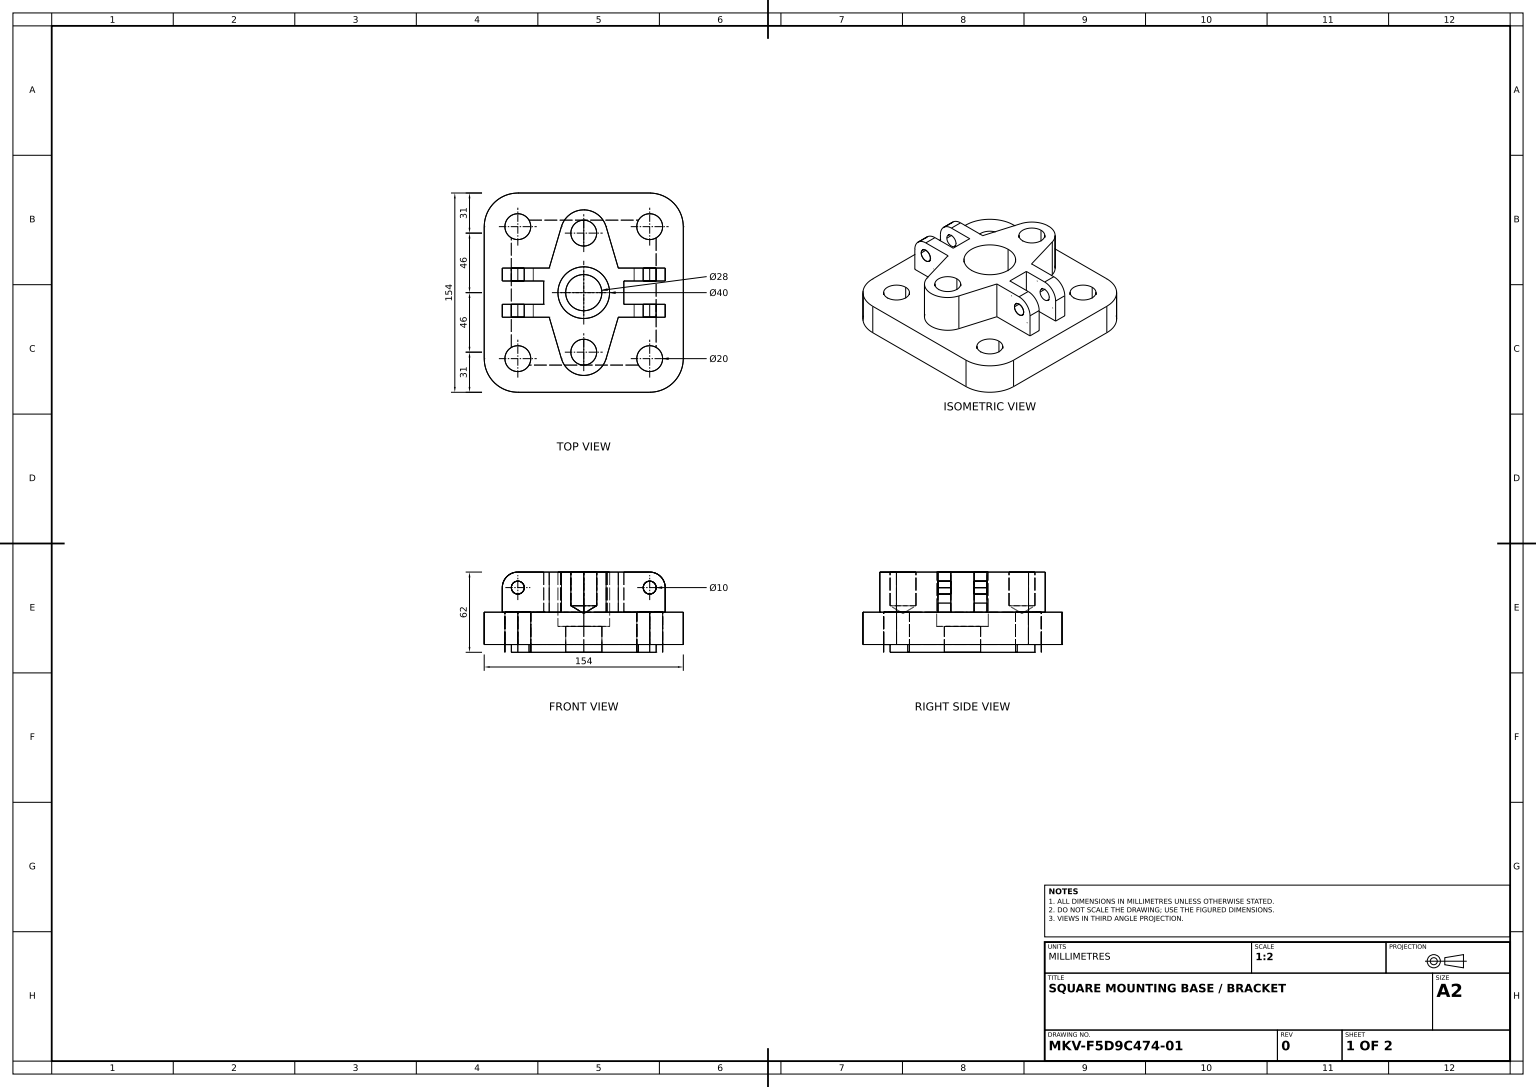
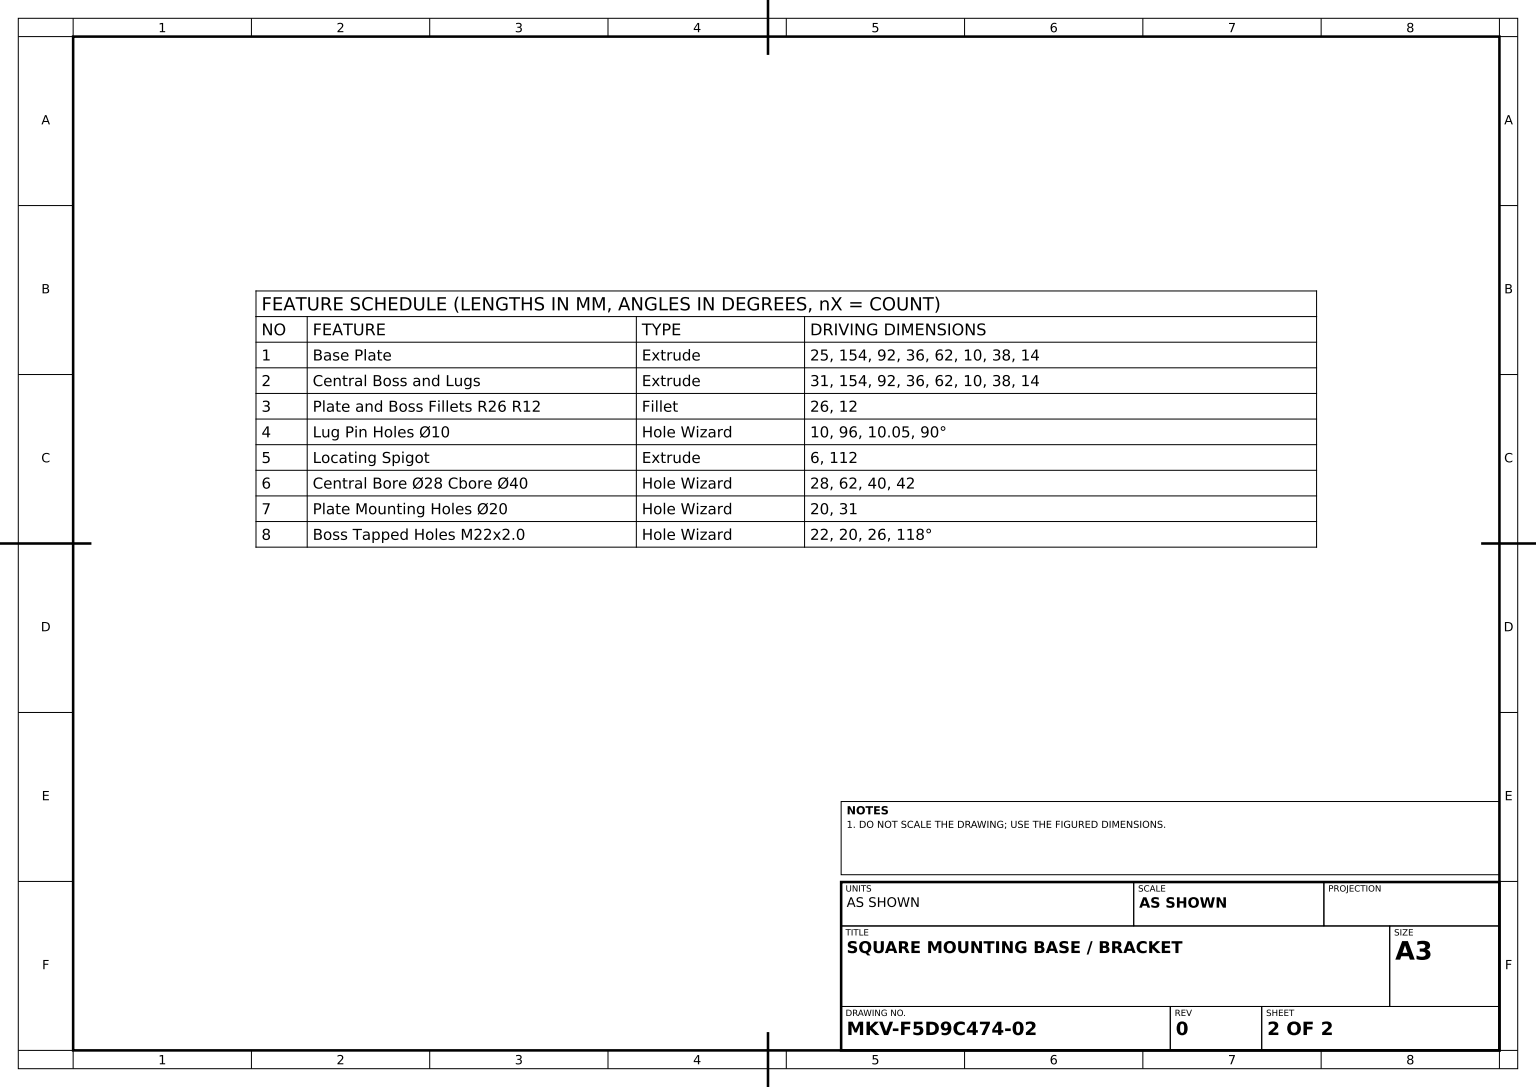
from build123d import *
from OCP.BRepFilletAPI import BRepFilletAPI_MakeFillet

# Parameters (mm, degrees)
PLATE_AND_BOSS_PROFILE_W             = 154
PLATE_AND_BOSS_PROFILE_H             = 154
PLATE_AND_BOSS_PROFILE_R             = 18
BASE_PLATE_DEPTH                     = 25
CENTRAL_START                        = 25
SKETCH1_3_R                          = 18
CENTRAL_BOSS_AND_LUGS_DEPTH          = 31
PLATE_AND_BOSS_FILLETS_R26_R12_R1    = 12
PLATE_AND_BOSS_FILLETS_R26_R12_R2    = 26
LUG_PIN_HOLES_10_D                   = 10
LUG_PIN_HOLES_10_CSINK_D             = 10.05
LUG_PIN_HOLES_10_CSINK_ANGLE         = 90
LOCATING_SPIGOT_PROFILE_112_W        = 112
LOCATING_SPIGOT_PROFILE_112_H        = 112
LOCATING_SPIGOT_DEPTH                = 6
CENTRAL_BORE_28_CBORE_40_D           = 28
CENTRAL_BORE_28_CBORE_40_CBORE_D     = 40
CENTRAL_BORE_28_CBORE_40_CBORE_DEPTH = 42
PLATE_MOUNTING_HOLES_20_D            = 20
BOSS_TAPPED_HOLES_M22X2_0_D          = 20
BOSS_TAPPED_HOLES_M22X2_0_DEPTH      = 26
BOSS_TAPPED_HOLES_M22X2_0_TIP        = 6.00860619


with BuildPart() as part:
    # Plate and Boss Profile → Base Plate (new body)
    # profile 1 of 4: a face of its own
    with BuildSketch(Plane(origin=(0, 0, 0), x_dir=(1, 0, 0), z_dir=(0, 1, 0))):
        Rectangle(PLATE_AND_BOSS_PROFILE_W, PLATE_AND_BOSS_PROFILE_H)
        with BuildLine():
            Line((-26.719653956, 19), (-17.266235066, 51.086956522))
            ThreePointArc((-17.266235066, 51.086956522), (0, 64), (17.266235066, 51.086956522))
            Line((17.266235066, 51.086956522), (26.719653956, 19))
            Line((26.719653956, 19), (63, 19))
            Line((63, 19), (63, 9))
            Line((63, 9), (31, 9))
            Line((31, 9), (31, -9))
            Line((31, -9), (63, -9))
            Line((63, -9), (63, -19))
            Line((63, -19), (26.719653956, -19))
            Line((26.719653956, -19), (17.266235066, -51.086956522))
            ThreePointArc((17.266235066, -51.086956522), (0, -64), (-17.266235066, -51.086956522))
            Line((-17.266235066, -51.086956522), (-26.719653956, -19))
            Line((-26.719653956, -19), (-63, -19))
            Line((-63, -19), (-63, -9))
            Line((-63, -9), (-31, -9))
            Line((-31, -9), (-31, 9))
            Line((-31, 9), (-63, 9))
            Line((-63, 9), (-63, 19))
            Line((-63, 19), (-26.719653956, 19))
        make_face(mode=Mode.SUBTRACT)
    # profile 2 of 4: a face of its own
    with BuildSketch(Plane(origin=(0, 0, 0), x_dir=(1, 0, 0), z_dir=(0, 1, 0))):
        with BuildLine():
            ThreePointArc((18, 46), (-2.569802406, 28.184385624), (-17.266235066, 51.086956522))
            Line((-17.266235066, 51.086956522), (-26.719653956, 19))
            Line((-26.719653956, 19), (-63, 19))
            Line((-63, 19), (-63, 9))
            Line((-63, 9), (-31, 9))
            Line((-31, 9), (-31, -9))
            Line((-31, -9), (-63, -9))
            Line((-63, -9), (-63, -19))
            Line((-63, -19), (-26.719653956, -19))
            Line((-26.719653956, -19), (-17.266235066, -51.086956522))
            ThreePointArc((-17.266235066, -51.086956522), (-2.569802406, -28.184385624), (18, -46))
            ThreePointArc((18, -46), (17.815614376, -48.569802406), (17.266235066, -51.086956522))
            Line((17.266235066, -51.086956522), (26.719653956, -19))
            Line((26.719653956, -19), (63, -19))
            Line((63, -19), (63, -9))
            Line((63, -9), (31, -9))
            Line((31, -9), (31, 9))
            Line((31, 9), (63, 9))
            Line((63, 9), (63, 19))
            Line((63, 19), (26.719653956, 19))
            Line((26.719653956, 19), (17.266235066, 51.086956522))
            ThreePointArc((17.266235066, 51.086956522), (17.815614376, 48.569802406), (18, 46))
        make_face()
    # profile 3 of 4: a face of its own
    with BuildSketch(Plane(origin=(0, 0, 0), x_dir=(1, 0, 0), z_dir=(0, 1, 0))):
        with Locations((0, 46)):
            Circle(PLATE_AND_BOSS_PROFILE_R)
    # profile 4 of 4: a face of its own
    with BuildSketch(Plane(origin=(0, 0, 0), x_dir=(1, 0, 0), z_dir=(0, 1, 0))):
        with Locations((0, -46)):
            Circle(PLATE_AND_BOSS_PROFILE_R)
    extrude(amount=BASE_PLATE_DEPTH)

    # Sketch1_3 → Central Boss and Lugs (add)
    with BuildSketch(Plane(origin=(0, 0, 0), x_dir=(1, 0, 0), z_dir=(0, 1, 0)).offset(CENTRAL_START)):
        with BuildLine():
            ThreePointArc((18, 46), (-2.569802406, 28.184385624), (-17.266235066, 51.086956522))
            Line((-17.266235066, 51.086956522), (-26.719653956, 19))
            Line((-26.719653956, 19), (-63, 19))
            Line((-63, 19), (-63, 9))
            Line((-63, 9), (-31, 9))
            Line((-31, 9), (-31, -9))
            Line((-31, -9), (-63, -9))
            Line((-63, -9), (-63, -19))
            Line((-63, -19), (-26.719653956, -19))
            Line((-26.719653956, -19), (-17.266235066, -51.086956522))
            ThreePointArc((-17.266235066, -51.086956522), (-2.569802406, -28.184385624), (18, -46))
            ThreePointArc((18, -46), (17.815614376, -48.569802406), (17.266235066, -51.086956522))
            Line((17.266235066, -51.086956522), (26.719653956, -19))
            Line((26.719653956, -19), (63, -19))
            Line((63, -19), (63, -9))
            Line((63, -9), (31, -9))
            Line((31, -9), (31, 9))
            Line((31, 9), (63, 9))
            Line((63, 9), (63, 19))
            Line((63, 19), (26.719653956, 19))
            Line((26.719653956, 19), (17.266235066, 51.086956522))
            ThreePointArc((17.266235066, 51.086956522), (17.815614376, 48.569802406), (18, 46))
        make_face()
        with Locations((0, 46)):
            Circle(SKETCH1_3_R)
        with Locations((0, -46)):
            Circle(SKETCH1_3_R)
    extrude(amount=CENTRAL_BOSS_AND_LUGS_DEPTH)

    # Plate and Boss Fillets R26 R12: one fillet with a radius per group of edges: ONE call of the kernel's fillet builder (fillet() takes one radius for all edges)
    plate_and_boss_fillets_r26_r12_edges_1 = [part.edges().sort_by_distance(p)[0] for p in [
        (63, 56, 14),
        (-63, 56, -14),
        (63, 56, -14),
        (-63, 56, 14),
    ]]
    plate_and_boss_fillets_r26_r12_edges_2 = [part.edges().sort_by_distance(p)[0] for p in [
        (77, 12.5, 77),
        (-77, 12.5, 77),
        (-77, 12.5, -77),
        (77, 12.5, -77),
    ]]
    plate_and_boss_fillets_r26_r12 = BRepFilletAPI_MakeFillet(part.part.solid().wrapped)
    for e in plate_and_boss_fillets_r26_r12_edges_1:
        plate_and_boss_fillets_r26_r12.Add(PLATE_AND_BOSS_FILLETS_R26_R12_R1, e.wrapped)
    for e in plate_and_boss_fillets_r26_r12_edges_2:
        plate_and_boss_fillets_r26_r12.Add(PLATE_AND_BOSS_FILLETS_R26_R12_R2, e.wrapped)
    add(Compound.cast(plate_and_boss_fillets_r26_r12.Shape()), mode=Mode.REPLACE)

    # Lug Pin Holes _10 (through all)
    with Locations(Plane.XY.offset(19)):
        with Locations((-51, 44), (51, 44)):
            CounterSinkHole(LUG_PIN_HOLES_10_D / 2, LUG_PIN_HOLES_10_CSINK_D / 2, counter_sink_angle=LUG_PIN_HOLES_10_CSINK_ANGLE)

    # Locating Spigot Profile _112 → Locating Spigot (add)
    with BuildSketch(Plane.XZ):
        Rectangle(LOCATING_SPIGOT_PROFILE_112_W, LOCATING_SPIGOT_PROFILE_112_H)
    extrude(amount=LOCATING_SPIGOT_DEPTH)

    # Central Bore _28 Cbore _40 (through all)
    with Locations(Plane(origin=(0, 56, 0), x_dir=(1, 0, 0), z_dir=(0, 1, 0))):
        with Locations((0, 0)):
            CounterBoreHole(CENTRAL_BORE_28_CBORE_40_D / 2, CENTRAL_BORE_28_CBORE_40_CBORE_D / 2, CENTRAL_BORE_28_CBORE_40_CBORE_DEPTH)

    # Plate Mounting Holes _20 (through all)
    with Locations(Plane(origin=(0, 25, 0), x_dir=(1, 0, 0), z_dir=(0, 1, 0))):
        with Locations((51, -51), (51, 51), (-51, 51), (-51, -51)):
            Hole(PLATE_MOUNTING_HOLES_20_D / 2)

    # Boss Tapped Holes M22x2.0
    with Locations(Plane(origin=(0, 56, 0), x_dir=(1, 0, 0), z_dir=(0, 1, 0))):
        with Locations((0, -46), (0, 46)):
            Hole(BOSS_TAPPED_HOLES_M22X2_0_D / 2, depth=BOSS_TAPPED_HOLES_M22X2_0_DEPTH)
            with Locations((0, 0, -(BOSS_TAPPED_HOLES_M22X2_0_DEPTH + BOSS_TAPPED_HOLES_M22X2_0_TIP / 2))):  # 118° drill point
                Cone(0, BOSS_TAPPED_HOLES_M22X2_0_D / 2, BOSS_TAPPED_HOLES_M22X2_0_TIP, mode=Mode.SUBTRACT)


solid = part.part
